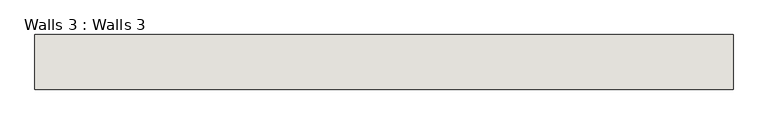
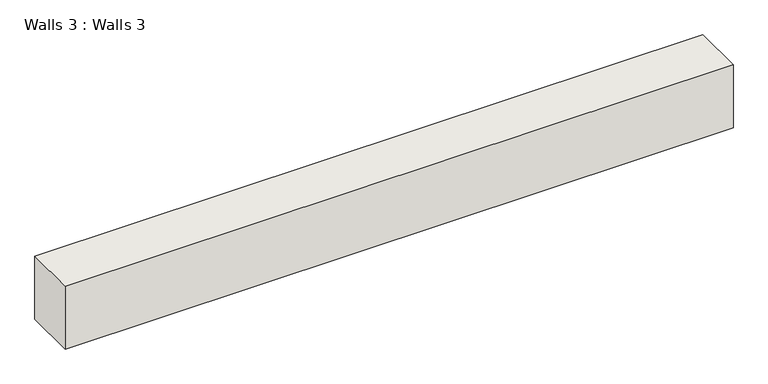
"""IFC4 building model written with IfcOpenShell, lengths in millimetres: wall geometry, Walls 3 : Walls 3."""

from ifc_helpers import new_model, si_unit, frame, origin, place, context, project, spatial, polyline, outline, extrude, source, transform, mapped, element, save


def walls_3_walls_3_34f02fba(model_context):
    return source(origin(), model_context, "Body", "SweptSolid", [
        extrude(outline(polyline([(-5234.779577, 1328.1827135), (-9130.6832287, 1328.1827135), (-9130.6832287, 1632.9827135), (-5234.779577, 1632.9827135), (-5234.779577, 1328.1827135)])), frame((0.0, 0.0, 7620.0), z_axis=(0.0, 0.0, 1.0), x_axis=(1.0, 0.0, 0.0)), (0.0, 0.0, 1.0), 387.9145619),
    ])


if __name__ == "__main__":
    model = new_model("IFC4")
    model_context = context("Model", 3, world=origin())
    ifc_project = project(units=[si_unit("LENGTHUNIT", "METRE", prefix="MILLI")], contexts=[model_context])
    site = spatial("IfcSite", under=ifc_project)
    building = spatial("IfcBuilding", under=site)
    placement = place(None, origin())
    walls_3_walls_3_shape = walls_3_walls_3_34f02fba(model_context)
    element("IfcWall", 1, ObjectType="Walls 3 : Walls 3", at=placement, inside=building, context=model_context, shape_type="MappedRepresentation", body=[
        mapped(walls_3_walls_3_shape, transform((0.0, 0.0, 0.0), x_axis=(1.0, 0.0, 0.0), y_axis=(0.0, 1.0, 0.0), z_axis=(0.0, 0.0, 1.0))),
    ])
    save(model, "model.ifc")

# Revit data of these elements
# Element 1 (IfcWall, "Walls 3 : Walls 3")
#   Materials on its faces: "Default Wall"
# Materials
#   "Default Wall": colour RGB 128 128 128, transparency 0
